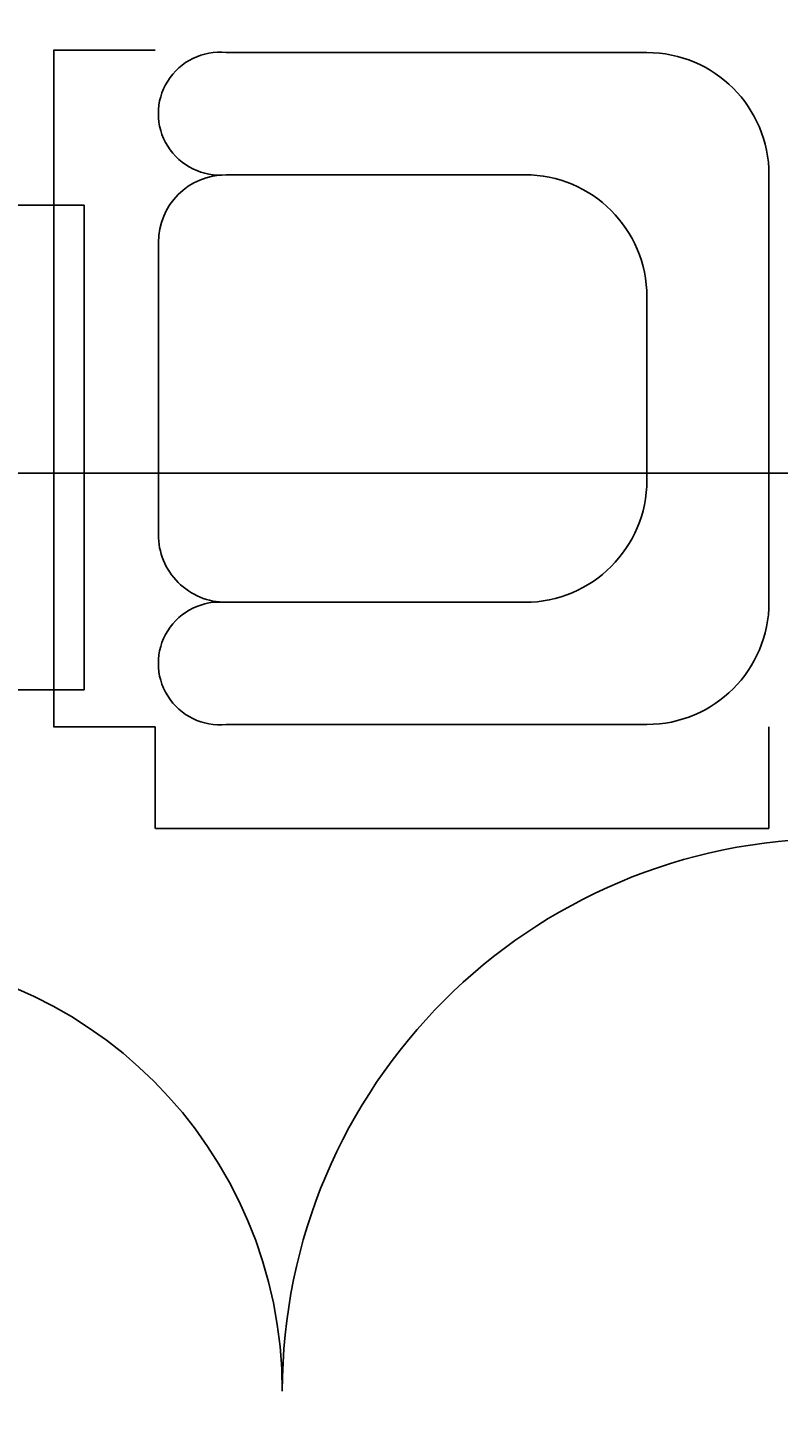
# Model space of a CAD drawing. Units: millimetres. Extents: x 19292 to 100733, y 12374 to 26974.
# Tile 13 of 24: x 29777 to 31036, y 14845 to 17195. Entities that reach past the tile are written whole.
import ezdxf

# ---------------------------------------------------------------- set-up
doc = ezdxf.new("R2010")
doc.units = ezdxf.units.MM
for name, color, linetype, lineweight in [('A-ANNO-DIMS', 2, 'Continuous', 18), ('A-DOOR', 4, 'Continuous', 25), ('A-FLOR-PATT', 252, 'Continuous', 13), ('A-FURN', 8, 'Continuous', 18)]:
    doc.layers.add(name, color=color, linetype=linetype, lineweight=lineweight)
doc.layers.add('FURNITURE', color=40, linetype='Continuous')
doc.styles.get("Standard").update_dxf_attribs({"font": 'arial.ttf'})
doc.dimstyles.get("Standard").update_dxf_attribs({"dimtxt": 0.18, "dimasz": 0.18, "dimexe": 0.18, "dimexo": 0.0625, "dimgap": 0.09, "dimtad": 0, "dimtih": 1, "dimtoh": 1, "dimdec": 4, "dimzin": 0, "dimdsep": 46, "dimtxsty": 'Standard', "dimcen": 0.09, "dimadec": 0, "dimazin": 0, "dimtfac": 1, "dimtdec": 4, "dimtofl": 0, "dimtmove": 0, "dimatfit": 3, "dimfxl": 1, "dimtolj": 1, "dimtzin": 0, "dimarcsym": 0})

# ---------------------------------------------------------------- blocks, each defined once
blk = doc.blocks.new('1sofa')
at = {"layer": 'FURNITURE'}
for p, q in [((9.45, 27), (-9.45, 27)), ((-14.85, 21.6), (-14.85, 3)), ((4.05, 21.6), (-4.05, 21.6)), ((14.85, 21.6), (14.85, 3)), ((-9.45, 16.2), (-9.45, 3)), ((9.45, 16.2), (9.45, 3)), ((6.45, 0), (-6.45, 0))]:
    blk.add_line(p, q, dxfattribs=at)
for centre, radius, start, end in [((-9.45, 21.6), 5.4, 90, 180), ((9.45, 21.6), 5.4, 0, 90), ((-4.05, 16.2), 5.4, 90, 180), ((4.05, 16.2), 5.4, 0, 90), ((-12.15, 2.715), 2.715, 173.97442, 6.02558), ((-6.45, 3), 3, 180, 270), ((6.45, 3), 3, 270, 0), ((12.15, 2.715), 2.715, 173.97442, 6.02558)]:
    blk.add_arc(centre, radius, start, end, dxfattribs=at)
blk = doc.blocks.new('*D47')
at = {"layer": 'A-ANNO-DIMS', "color": 0, "lineweight": -2, "transparency": 16777216}
for p, q in [((29749.2, 16897.5), (29871.3, 16897.5)), ((29871.2, 16897.4), (29871.2, 16490.9)), ((29871.2, 16084), (29871.2, 16490.5)), ((29749.2, 16083.8), (29871.3, 16083.8))]:
    blk.add_line(p, q, dxfattribs=at)
at = {"layer": 'A-ANNO-DIMS', "color": 0, "transparency": 16777216}
for points in [[(29871.1, 16897.4), (29871.2, 16897.4), (29871.2, 16897.5)], [(29871.1, 16084), (29871.2, 16084), (29871.2, 16083.8)]]:
    blk.add_solid(points, dxfattribs=at)
at = {"layer": 'Defpoints', "color": 0, "transparency": 16777216}
for p in [(29749.1, 16897.5), (29871.2, 16897.5), (29749.1, 16083.8)]:
    blk.add_point(p, dxfattribs=at)
at = {"layer": 'A-ANNO-DIMS', "color": 0, "transparency": 16777216, "insert": (29871.2, 16490.7), "char_height": 0.18, "attachment_point": 5}
blk.add_mtext('\\A1;814 TYP.', dxfattribs=at)
blk = doc.blocks.new('*D48')
at = {"layer": 'A-ANNO-DIMS', "color": 0, "lineweight": -2, "transparency": 16777216}
for p, q in [((29990.3, 17158), (29819.7, 17158)), ((29819.9, 17157.9), (29819.9, 16590)), ((29819.9, 16021.8), (29819.9, 16589.6)), ((29990.3, 16021.6), (29819.7, 16021.6))]:
    blk.add_line(p, q, dxfattribs=at)
at = {"layer": 'A-ANNO-DIMS', "color": 0, "transparency": 16777216}
for points in [[(29819.9, 17157.9), (29820, 17157.9), (29819.9, 17158)], [(29819.9, 16021.8), (29820, 16021.8), (29819.9, 16021.6)]]:
    blk.add_solid(points, dxfattribs=at)
at = {"layer": 'Defpoints', "color": 0, "transparency": 16777216}
for p in [(29990.4, 17158), (29819.9, 16021.6), (29990.4, 16021.6)]:
    blk.add_point(p, dxfattribs=at)
at = {"layer": 'A-ANNO-DIMS', "color": 0, "transparency": 16777216, "insert": (29819.9, 16589.8), "char_height": 0.18, "attachment_point": 5}
blk.add_mtext('\\A1;ARMCHAIR 1136', dxfattribs=at)
blk = doc.blocks.new('*D49')
at = {"layer": 'A-ANNO-DIMS', "color": 0, "lineweight": -2, "transparency": 16777216}
for p, q in [((29990.4, 16021.6), (29990.4, 15851)), ((31021.2, 16021.6), (31021.2, 15851)), ((29990.6, 15851.2), (30505.5, 15851.2)), ((31021, 15851.2), (30506.1, 15851.2))]:
    blk.add_line(p, q, dxfattribs=at)
at = {"layer": 'A-ANNO-DIMS', "color": 0, "transparency": 16777216}
for points in [[(29990.6, 15851.2), (29990.6, 15851.1), (29990.4, 15851.2)], [(31021, 15851.2), (31021, 15851.1), (31021.2, 15851.2)]]:
    blk.add_solid(points, dxfattribs=at)
at = {"layer": 'Defpoints', "color": 0, "transparency": 16777216}
for p in [(29990.4, 16021.6), (31021.2, 16021.6), (31021.2, 15851.2)]:
    blk.add_point(p, dxfattribs=at)
at = {"layer": 'A-ANNO-DIMS', "color": 0, "transparency": 16777216, "insert": (30505.8, 15851.2), "char_height": 0.18, "attachment_point": 5}
blk.add_mtext('\\A1;1031', dxfattribs=at)
blk = doc.blocks.new('*D70')
at = {"layer": 'A-ANNO-DIMS', "color": 0, "lineweight": -2, "transparency": 16777216}
for p, q in [((23573.9, 17387.7), (36879.3, 17387.7)), ((36879.2, 17387.6), (36879.2, 16917.9)), ((36879.2, 16447.9), (36879.2, 16917.6)), ((23573.9, 16447.7), (36879.3, 16447.7))]:
    blk.add_line(p, q, dxfattribs=at)
at = {"layer": 'A-ANNO-DIMS', "color": 0, "transparency": 16777216}
for points in [[(36879.1, 17387.6), (36879.2, 17387.6), (36879.2, 17387.7)], [(36879.1, 16447.9), (36879.2, 16447.9), (36879.2, 16447.7)]]:
    blk.add_solid(points, dxfattribs=at)
at = {"layer": 'Defpoints', "color": 0, "transparency": 16777216}
for p in [(23573.8, 17387.7), (36879.2, 17387.7), (23573.8, 16447.7)]:
    blk.add_point(p, dxfattribs=at)
at = {"layer": 'A-ANNO-DIMS', "color": 0, "transparency": 16777216, "insert": (36879.2, 16917.7), "char_height": 0.18, "attachment_point": 5}
blk.add_mtext('\\A1;940', dxfattribs=at)
blk = doc.blocks.new('*D79')
at = {"layer": 'A-ANNO-DIMS', "color": 0, "lineweight": -2, "transparency": 16777216}
for p, q in [((22694.1, 22860.7), (22694.1, 12808.8)), ((36144.2, 15985.7), (36144.2, 12808.8)), ((22694.3, 12809), (29418.7, 12809)), ((36144, 12809), (29419.6, 12809))]:
    blk.add_line(p, q, dxfattribs=at)
at = {"layer": 'A-ANNO-DIMS', "color": 0, "transparency": 16777216}
for points in [[(22694.3, 12809), (22694.3, 12809), (22694.1, 12809)], [(36144, 12809), (36144, 12809), (36144.2, 12809)]]:
    blk.add_solid(points, dxfattribs=at)
at = {"layer": 'Defpoints', "color": 0, "transparency": 16777216}
for p in [(22694.1, 22860.7), (36144.2, 15985.7), (36144.2, 12809)]:
    blk.add_point(p, dxfattribs=at)
at = {"layer": 'A-ANNO-DIMS', "color": 0, "transparency": 16777216, "insert": (29419.2, 12809), "char_height": 0.18, "attachment_point": 5}
blk.add_mtext('\\A1;13450', dxfattribs=at)
blk = doc.blocks.new('*D82')
at = {"layer": 'A-ANNO-DIMS', "color": 0, "lineweight": -2, "transparency": 16777216}
for p, q in [((27198.8, 13562.8), (27198.8, 23555.9)), ((27199, 23555.7), (29296.4, 23555.7)), ((31394.6, 23555.7), (29297.2, 23555.7)), ((31394.8, 13544.1), (31394.8, 23555.9))]:
    blk.add_line(p, q, dxfattribs=at)
at = {"layer": 'A-ANNO-DIMS', "color": 0, "transparency": 16777216}
for points in [[(27199, 23555.8), (27199, 23555.7), (27198.8, 23555.7)], [(31394.6, 23555.8), (31394.6, 23555.7), (31394.8, 23555.7)]]:
    blk.add_solid(points, dxfattribs=at)
at = {"layer": 'Defpoints', "color": 0, "transparency": 16777216}
for p in [(31394.8, 23555.7), (27198.8, 13562.7), (31394.8, 13544)]:
    blk.add_point(p, dxfattribs=at)
at = {"layer": 'A-ANNO-DIMS', "color": 0, "transparency": 16777216, "insert": (29296.8, 23555.7), "char_height": 0.18, "attachment_point": 5}
blk.add_mtext('\\A1;4196', dxfattribs=at)
blk = doc.blocks.new('*D86')
at = {"layer": 'A-ANNO-DIMS', "color": 0, "lineweight": -2, "transparency": 16777216}
for p, q in [((27198.8, 15132.8), (27198.8, 23555.9)), ((27199, 23555.7), (29198.5, 23555.7)), ((31198.6, 23555.7), (29199.2, 23555.7)), ((31198.8, 15132.8), (31198.8, 23555.9))]:
    blk.add_line(p, q, dxfattribs=at)
at = {"layer": 'A-ANNO-DIMS', "color": 0, "transparency": 16777216}
for points in [[(27199, 23555.8), (27199, 23555.7), (27198.8, 23555.7)], [(31198.6, 23555.8), (31198.6, 23555.7), (31198.8, 23555.7)]]:
    blk.add_solid(points, dxfattribs=at)
at = {"layer": 'Defpoints', "color": 0, "transparency": 16777216}
for p in [(31198.8, 23555.7), (27198.8, 15132.7), (31198.8, 15132.7)]:
    blk.add_point(p, dxfattribs=at)
at = {"layer": 'A-ANNO-DIMS', "color": 0, "transparency": 16777216, "insert": (29198.8, 23555.7), "char_height": 0.18, "attachment_point": 5}
blk.add_mtext('\\A1;4000', dxfattribs=at)

msp = doc.modelspace()

# ---------------------------------------------------------------- hatches: boundary and pattern name
at = {"layer": 'A-FLOR-PATT'}
h = msp.add_hatch(dxfattribs=at)
h.set_pattern_fill('CROSS', color=256, scale=40)
h.paths.add_polyline_path([(36144.169, 19010.725), (33719.169, 19010.725), (33719.169, 18850.725), (33719.169, 18003.026), (33719.169, 15985.725), (36144.169, 15985.725)])
h.paths.add_polyline_path([(36144.132, 22460.725), (34419.132, 22460.725), (34419.132, 22208.026, -0.34415073), (35121.831, 21308.026), (34419.132, 21308.026), (34419.132, 21260.725), (36144.132, 21260.725)])
h.paths.add_polyline_path([(34419.132, 22208.026), (34419.132, 21388.026), (35118.375, 21388.026, 0.32018294)], flags=17)
h.paths.add_polyline_path([(31169.132, 22460.725), (28369.132, 22460.725), (28369.132, 21460.725), (31169.132, 21460.725)])
h.paths.add_polyline_path([(34010.406, 17316.149), (36018.156, 17316.149), (36018.156, 17722.778), (34010.406, 17722.778)], flags=24)
h.paths.add_polyline_path([(34456.896, 21920.301), (35605.434, 21920.301), (35605.434, 22313.518), (34456.896, 22313.518)], flags=25)
h.paths.add_polyline_path([(29263.068, 21823.707), (30421.489, 21823.707), (30421.489, 22034.008), (29263.068, 22034.008)], flags=24)
h = msp.add_hatch(dxfattribs=at)
h.set_pattern_fill('CROSS', color=256, scale=40)
h.paths.add_polyline_path([(31394.799, 14906.403), (31051.542, 14906.403), (29468.571, 14906.403), (27198.815, 14906.403), (27198.815, 13543.993), (31394.799, 13543.993)])
h.paths.add_polyline_path([(27828.096, 14036.581), (30629.164, 14036.581), (30629.164, 14443.478), (27828.096, 14443.478)], flags=24)

# ---------------------------------------------------------------- linework, layer by layer
at = {"layer": 'A-DOOR'}
for centre, radius, start, end in [((31131.542, 14906.403), 927.699, 90, 180), ((29468.571, 14906.403), 735.272, 0, 90)]:
    msp.add_arc(centre, radius, start, end, dxfattribs=at)

# ---------------------------------------------------------------- block references
at = {"layer": 'A-FURN', "xscale": 37.98437848243485, "yscale": 37.98437848243485, "zscale": 37.98437848243485, "rotation": 270}
msp.add_blockref('1sofa', (29995.613, 16589.824), dxfattribs=at)

# ---------------------------------------------------------------- dimensions: what is measured, and where the dimension line sits
at = {"layer": 'A-ANNO-DIMS'}
for base, p1, p2, override, picture, middle in [((31394.799, 23555.725), (27198.815, 13562.748), (31394.799, 13543.993), {"dimdec": 0, "dimlfac": 1, "dimrnd": 0, "dimzin": 0, "dimdsep": 46, "dimlunit": 2}, '*D82', (29296.807, 23555.725)), ((31198.815, 23555.725), (27198.815, 15132.748), (31198.815, 15132.748), {"dimdec": 0, "dimlfac": 1, "dimrnd": 0, "dimzin": 0, "dimdsep": 46, "dimlunit": 2}, '*D86', (29198.815, 23555.725)), ((36144.169, 12808.993), (22694.132, 22860.725), (36144.169, 15985.725), {"dimdec": 0, "dimlfac": 1, "dimrnd": 0, "dimzin": 0, "dimdsep": 46, "dimlunit": 2}, '*D79', (29419.151, 12808.993)), ((31021.192, 15851.153), (29990.387, 16021.616), (31021.192, 16021.616), {"dimdec": 0, "dimrnd": 0, "dimzin": 0, "dimlunit": 2}, '*D49', (30505.789, 15851.153))]:
    dim = msp.add_linear_dim(base=base, p1=p1, p2=p2, dimstyle='Standard', override=override, dxfattribs=at)
    dim.commit()
    dim.dimension.update_dxf_attribs({"geometry": picture, "text_midpoint": middle})
dim = msp.add_linear_dim(base=(36879.169, 17387.748), p1=(23573.815, 16447.748), p2=(23573.815, 17387.748), angle=90, dimstyle='Standard', override={"dimdec": 0, "dimlfac": 1, "dimrnd": 0, "dimzin": 0, "dimdsep": 46, "dimlunit": 2}, dxfattribs=at)
dim.commit()
dim.dimension.update_dxf_attribs({"geometry": '*D70', "text_midpoint": (36879.169, 16917.748)})
for base, p1, p2, angle, text, picture, middle in [((29819.925, 16021.616), (29990.387, 17158.032), (29990.387, 16021.616), 270, 'ARMCHAIR <>', '*D48', (29819.925, 16589.824)), ((29871.169, 16897.53), (29749.113, 16083.823), (29749.113, 16897.53), 90, '<> TYP.', '*D47', (29871.169, 16490.677))]:
    dim = msp.add_linear_dim(base=base, p1=p1, p2=p2, angle=angle, text=text, dimstyle='Standard', override={"dimdec": 0, "dimrnd": 0, "dimzin": 0, "dimlunit": 2}, dxfattribs=at)
    dim.commit()
    dim.dimension.update_dxf_attribs({"geometry": picture, "text_midpoint": middle})

doc.saveas('drawing.dxf')
